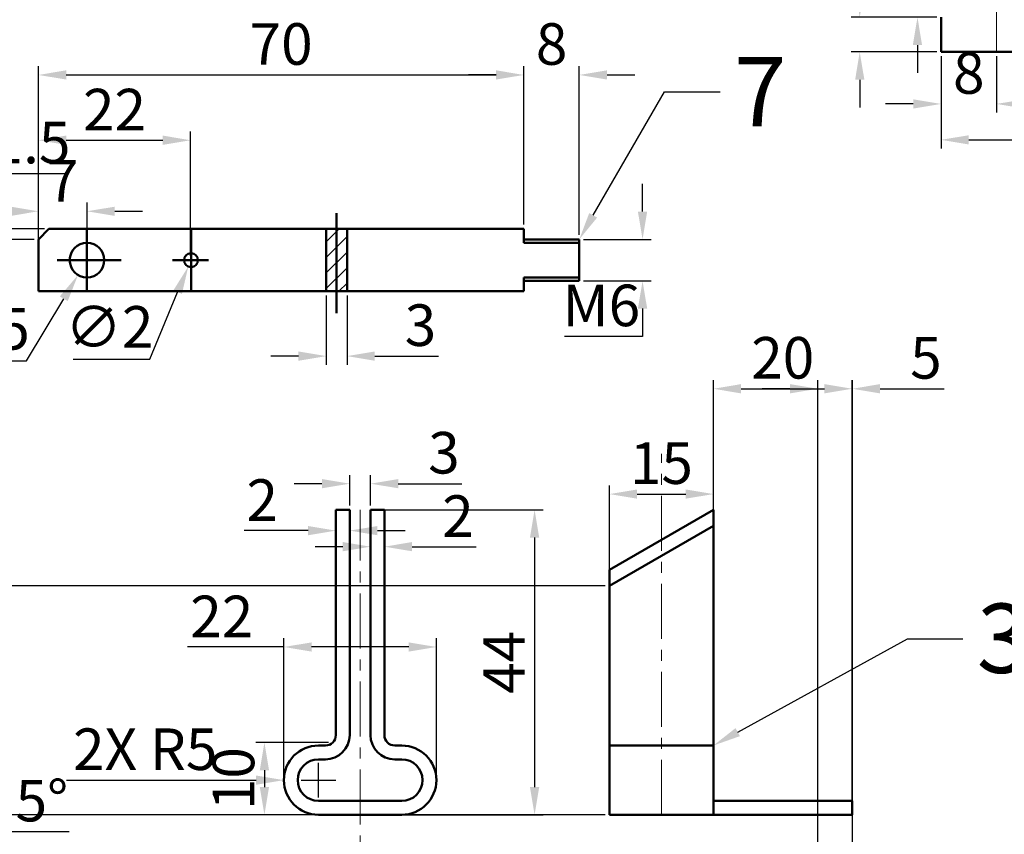
# Model space of a CAD drawing. Units: millimetres. Extents: x 1145 to 1687, y 12 to 400.
# Tile 3 of 6: x 1274 to 1416, y 168 to 285. Entities that reach past the tile are written whole.
import ezdxf
from ezdxf import colors
from ezdxf.entities.mleader import LeaderData, LeaderLine
from ezdxf.math import Vec2, Vec3

# ---------------------------------------------------------------- set-up
doc = ezdxf.new("R2010")
doc.units = ezdxf.units.MM
doc.header["$LTSCALE"] = 0.5
doc.linetypes.add('CENTER', pattern=[50.8, 31.75, -6.35, 6.35, -6.35])
for name, color, linetype, lineweight in [('M-CNTR', 1, 'CENTER', 18), ('M-DIMS', 2, 'Continuous', 25), ('M-HATC', 8, 'Continuous', 18), ('M-OUTL', 7, 'Continuous', 50), ('M-TEXT', 3, 'Continuous', 25)]:
    doc.layers.add(name, color=color, linetype=linetype, lineweight=lineweight)
doc.styles.get("Standard").update_dxf_attribs({"font": 'arial.ttf'})
doc.dimstyles.new('ISO-25', dxfattribs={"dimtxt": 6, "dimasz": 4, "dimexe": 1.25, "dimexo": 0.625, "dimtad": 1, "dimtoh": 1, "dimdec": 0, "dimtxsty": 'Standard', "dimcen": 2.5, "dimadec": 0, "dimazin": 0, "dimtfac": 1, "dimtdec": 0, "dimtofl": 0, "dimtmove": 0, "dimatfit": 3, "dimfxl": 1, "dimarcsym": 0})

# ---------------------------------------------------------------- blocks, each defined once
blk = doc.blocks.new('*D33')
at = {"layer": 'Defpoints', "color": 0, "ltscale": 0.5, "transparency": 16777216}
for p in [(1354.69, 277.15), (1346.69, 254.93), (1354.69, 253.43)]:
    blk.add_point(p, dxfattribs=at)
at = {"layer": 'M-DIMS', "color": 0, "lineweight": -2, "ltscale": 0.5, "transparency": 16777216}
for p, q in [((1346.69, 255.56), (1346.69, 278.4)), ((1354.69, 254.06), (1354.69, 278.4)), ((1342.69, 277.15), (1338.69, 277.15)), ((1358.69, 277.15), (1362.69, 277.15))]:
    blk.add_line(p, q, dxfattribs=at)
at = {"layer": 'M-DIMS', "color": 0, "ltscale": 0.5, "transparency": 16777216}
for points in [[(1342.69, 277.82), (1342.69, 276.49), (1346.69, 277.15)], [(1358.69, 277.82), (1358.69, 276.49), (1354.69, 277.15)]]:
    blk.add_solid(points, dxfattribs=at)
at = {"layer": 'M-DIMS', "color": 0, "ltscale": 0.5, "transparency": 16777216, "insert": (1350.69, 280.84), "char_height": 6, "attachment_point": 5}
blk.add_mtext('8', dxfattribs=at)
blk = doc.blocks.new('*D34')
at = {"layer": 'Defpoints', "color": 0, "ltscale": 0.5, "transparency": 16777216}
for p in [(1283.69, 257.48), (1283.69, 250.43), (1276.69, 249.68)]:
    blk.add_point(p, dxfattribs=at)
at = {"layer": 'M-DIMS', "color": 0, "lineweight": -2, "ltscale": 0.5, "transparency": 16777216}
for p, q in [((1276.69, 250.31), (1276.69, 258.73)), ((1283.69, 251.06), (1283.69, 258.73)), ((1272.69, 257.48), (1268.69, 257.48)), ((1287.69, 257.48), (1291.69, 257.48))]:
    blk.add_line(p, q, dxfattribs=at)
at = {"layer": 'M-DIMS', "color": 0, "ltscale": 0.5, "transparency": 16777216}
for points in [[(1272.69, 258.14), (1272.69, 256.81), (1276.69, 257.48)], [(1287.69, 258.14), (1287.69, 256.81), (1283.69, 257.48)]]:
    blk.add_solid(points, dxfattribs=at)
at = {"layer": 'M-DIMS', "color": 0, "ltscale": 0.5, "transparency": 16777216, "insert": (1280.19, 261.1), "char_height": 6, "attachment_point": 5}
blk.add_mtext('7', dxfattribs=at)
blk = doc.blocks.new('*D35')
at = {"layer": 'Defpoints', "color": 0, "ltscale": 0.5, "transparency": 16777216}
for p in [(1298.62, 267.73), (1298.62, 250.43), (1276.69, 249.68)]:
    blk.add_point(p, dxfattribs=at)
at = {"layer": 'M-DIMS', "color": 0, "lineweight": -2, "ltscale": 0.5, "transparency": 16777216}
for p, q in [((1276.69, 250.31), (1276.69, 268.98)), ((1298.62, 251.06), (1298.62, 268.98)), ((1280.69, 267.73), (1294.62, 267.73))]:
    blk.add_line(p, q, dxfattribs=at)
at = {"layer": 'M-DIMS', "color": 0, "ltscale": 0.5, "transparency": 16777216}
for points in [[(1280.69, 268.4), (1280.69, 267.06), (1276.69, 267.73)], [(1294.62, 268.4), (1294.62, 267.06), (1298.62, 267.73)]]:
    blk.add_solid(points, dxfattribs=at)
at = {"layer": 'M-DIMS', "color": 0, "ltscale": 0.5, "transparency": 16777216, "insert": (1287.66, 271.37), "char_height": 6, "attachment_point": 5}
blk.add_mtext('22', dxfattribs=at)
blk = doc.blocks.new('*D36')
at = {"layer": 'Defpoints', "color": 0, "ltscale": 0.5, "transparency": 16777216}
for p in [(1346.69, 277.15), (1346.69, 254.93), (1276.69, 249.68)]:
    blk.add_point(p, dxfattribs=at)
at = {"layer": 'M-DIMS', "color": 0, "lineweight": -2, "ltscale": 0.5, "transparency": 16777216}
for p, q in [((1276.69, 250.31), (1276.69, 278.4)), ((1346.69, 255.56), (1346.69, 278.4)), ((1280.69, 277.15), (1342.69, 277.15))]:
    blk.add_line(p, q, dxfattribs=at)
at = {"layer": 'M-DIMS', "color": 0, "ltscale": 0.5, "transparency": 16777216}
for points in [[(1280.69, 277.82), (1280.69, 276.49), (1276.69, 277.15)], [(1342.69, 277.82), (1342.69, 276.49), (1346.69, 277.15)]]:
    blk.add_solid(points, dxfattribs=at)
at = {"layer": 'M-DIMS', "color": 0, "ltscale": 0.5, "transparency": 16777216, "insert": (1311.69, 280.84), "char_height": 6, "attachment_point": 5}
blk.add_mtext('70', dxfattribs=at)
blk = doc.blocks.new('*D37')
at = {"layer": 'Defpoints', "color": 0, "ltscale": 0.5, "transparency": 16777216}
for p in [(1354.69, 253.43), (1354.69, 247.43), (1363.81, 247.43)]:
    blk.add_point(p, dxfattribs=at)
at = {"layer": 'M-DIMS', "color": 0, "lineweight": -2, "ltscale": 0.5, "transparency": 16777216}
for p, q in [((1363.81, 257.43), (1363.81, 261.43)), ((1355.31, 253.43), (1365.06, 253.43)), ((1355.31, 247.43), (1365.06, 247.43)), ((1363.81, 243.43), (1363.81, 239.43)), ((1363.81, 239.43), (1352.55, 239.43))]:
    blk.add_line(p, q, dxfattribs=at)
at = {"layer": 'M-DIMS', "color": 0, "ltscale": 0.5, "transparency": 16777216}
for points in [[(1363.14, 257.43), (1364.48, 257.43), (1363.81, 253.43)], [(1363.14, 243.43), (1364.48, 243.43), (1363.81, 247.43)]]:
    blk.add_solid(points, dxfattribs=at)
at = {"layer": 'M-DIMS', "color": 0, "ltscale": 0.5, "transparency": 16777216, "insert": (1357.87, 243.12), "char_height": 6, "attachment_point": 5}
blk.add_mtext('M6', dxfattribs=at)
blk = doc.blocks.new('*D38')
at = {"layer": 'Defpoints', "color": 0, "ltscale": 0.5, "transparency": 16777216}
for p in [(1318.19, 245.93), (1321.19, 245.93), (1321.19, 236.58)]:
    blk.add_point(p, dxfattribs=at)
at = {"layer": 'M-DIMS', "color": 0, "lineweight": -2, "ltscale": 0.5, "transparency": 16777216}
for p, q in [((1318.19, 245.31), (1318.19, 235.33)), ((1321.19, 245.31), (1321.19, 235.33)), ((1314.19, 236.58), (1310.19, 236.58)), ((1325.19, 236.58), (1334.37, 236.58))]:
    blk.add_line(p, q, dxfattribs=at)
at = {"layer": 'M-DIMS', "color": 0, "ltscale": 0.5, "transparency": 16777216}
for points in [[(1314.19, 237.25), (1314.19, 235.91), (1318.19, 236.58)], [(1325.19, 237.25), (1325.19, 235.91), (1321.19, 236.58)]]:
    blk.add_solid(points, dxfattribs=at)
at = {"layer": 'M-DIMS', "color": 0, "ltscale": 0.5, "transparency": 16777216, "insert": (1331.78, 240.27), "char_height": 6, "attachment_point": 5}
blk.add_mtext('3', dxfattribs=at)
blk = doc.blocks.new('*D39')
at = {"layer": 'Defpoints', "color": 0, "ltscale": 0.5, "transparency": 16777216}
for p in [(1299.07, 251.35), (1298.3, 249.51)]:
    blk.add_point(p, dxfattribs=at)
at = {"layer": 'M-DIMS', "color": 0, "lineweight": -2, "ltscale": 0.5, "transparency": 16777216}
for p, q in [((1298.69, 247.93), (1298.69, 252.93)), ((1296.19, 250.43), (1301.19, 250.43)), ((1292.74, 236.16), (1296.76, 245.82)), ((1281.71, 236.16), (1292.74, 236.16))]:
    blk.add_line(p, q, dxfattribs=at)
at = {"layer": 'M-DIMS', "color": 0, "ltscale": 0.5, "transparency": 16777216}
blk.add_solid([(1296.15, 246.07), (1297.38, 245.56), (1298.3, 249.51)], dxfattribs=at)
at = {"layer": 'M-DIMS', "color": 0, "ltscale": 0.5, "transparency": 16777216, "insert": (1286.91, 240.02), "char_height": 6, "attachment_point": 5}
blk.add_mtext('∅2', dxfattribs=at)
blk = doc.blocks.new('*D40')
at = {"layer": 'Defpoints', "color": 0, "ltscale": 0.5, "transparency": 16777216}
for p in [(1284.98, 252.57), (1282.4, 248.29)]:
    blk.add_point(p, dxfattribs=at)
at = {"layer": 'M-DIMS', "color": 0, "lineweight": -2, "ltscale": 0.5, "transparency": 16777216}
for p, q in [((1283.69, 247.93), (1283.69, 252.93)), ((1281.19, 250.43), (1286.19, 250.43)), ((1274.96, 235.89), (1280.34, 244.86)), ((1263.83, 235.89), (1274.96, 235.89))]:
    blk.add_line(p, q, dxfattribs=at)
at = {"layer": 'M-DIMS', "color": 0, "ltscale": 0.5, "transparency": 16777216}
blk.add_solid([(1279.77, 245.2), (1280.91, 244.52), (1282.4, 248.29)], dxfattribs=at)
at = {"layer": 'M-DIMS', "color": 0, "ltscale": 0.5, "transparency": 16777216, "insert": (1269.08, 239.75), "char_height": 6, "attachment_point": 5}
blk.add_mtext('∅5', dxfattribs=at)
blk = doc.blocks.new('*D41')
at = {"layer": 'Defpoints', "color": 0, "ltscale": 0.5, "transparency": 16777216}
for p in [(1406.86, 280.47), (1456.86, 280.47), (1456.86, 267.79)]:
    blk.add_point(p, dxfattribs=at)
at = {"layer": 'M-DIMS', "color": 0, "lineweight": -2, "ltscale": 0.5, "transparency": 16777216}
for p, q in [((1406.86, 279.85), (1406.86, 266.54)), ((1456.86, 279.85), (1456.86, 266.54)), ((1410.86, 267.79), (1452.86, 267.79))]:
    blk.add_line(p, q, dxfattribs=at)
at = {"layer": 'M-DIMS', "color": 0, "ltscale": 0.5, "transparency": 16777216}
for points in [[(1410.86, 268.45), (1410.86, 267.12), (1406.86, 267.79)], [(1452.86, 268.45), (1452.86, 267.12), (1456.86, 267.79)]]:
    blk.add_solid(points, dxfattribs=at)
at = {"layer": 'M-DIMS', "color": 0, "ltscale": 0.5, "transparency": 16777216, "insert": (1431.86, 271.48), "char_height": 6, "attachment_point": 5}
blk.add_mtext('50', dxfattribs=at)
blk = doc.blocks.new('*D42')
at = {"layer": 'Defpoints', "color": 0, "ltscale": 0.5, "transparency": 16777216}
for p in [(1406.86, 280.47), (1414.86, 280.47), (1414.86, 272.97)]:
    blk.add_point(p, dxfattribs=at)
at = {"layer": 'M-DIMS', "color": 0, "lineweight": -2, "ltscale": 0.5, "transparency": 16777216}
for p, q in [((1406.86, 279.85), (1406.86, 271.72)), ((1414.86, 279.85), (1414.86, 271.72)), ((1402.86, 272.97), (1398.86, 272.97)), ((1418.86, 272.97), (1422.86, 272.97))]:
    blk.add_line(p, q, dxfattribs=at)
at = {"layer": 'M-DIMS', "color": 0, "ltscale": 0.5, "transparency": 16777216}
for points in [[(1402.86, 273.63), (1402.86, 272.3), (1406.86, 272.97)], [(1418.86, 273.63), (1418.86, 272.3), (1414.86, 272.97)]]:
    blk.add_solid(points, dxfattribs=at)
at = {"layer": 'M-DIMS', "color": 0, "ltscale": 0.5, "transparency": 16777216, "insert": (1410.86, 276.66), "char_height": 6, "attachment_point": 5}
blk.add_mtext('8', dxfattribs=at)
blk = doc.blocks.new('*D43')
at = {"layer": 'Defpoints', "color": 0, "ltscale": 0.5, "transparency": 16777216}
for p in [(1395.13, 285.47), (1406.86, 285.47), (1406.86, 280.47)]:
    blk.add_point(p, dxfattribs=at)
at = {"layer": 'M-DIMS', "color": 0, "lineweight": -2, "ltscale": 0.5, "transparency": 16777216}
for p, q in [((1395.13, 289.47), (1395.13, 293.47)), ((1395.13, 293.47), (1399.74, 293.47)), ((1406.23, 285.47), (1393.88, 285.47)), ((1406.23, 280.47), (1393.88, 280.47)), ((1395.13, 276.47), (1395.13, 272.47))]:
    blk.add_line(p, q, dxfattribs=at)
at = {"layer": 'M-DIMS', "color": 0, "ltscale": 0.5, "transparency": 16777216}
for points in [[(1394.47, 289.47), (1395.8, 289.47), (1395.13, 285.47)], [(1394.47, 276.47), (1395.8, 276.47), (1395.13, 280.47)]]:
    blk.add_solid(points, dxfattribs=at)
at = {"layer": 'M-DIMS', "color": 0, "ltscale": 0.5, "transparency": 16777216, "insert": (1397.75, 297.15), "char_height": 6, "attachment_point": 5}
blk.add_mtext('5', dxfattribs=at)
blk = doc.blocks.new('*D44')
at = {"layer": 'Defpoints', "color": 0, "ltscale": 0.5, "transparency": 16777216}
for p in [(1403.46, 290.47), (1414.86, 290.47), (1406.86, 285.47)]:
    blk.add_point(p, dxfattribs=at)
at = {"layer": 'M-DIMS', "color": 0, "lineweight": -2, "ltscale": 0.5, "transparency": 16777216}
for p, q in [((1403.46, 294.47), (1403.46, 298.47)), ((1403.46, 298.47), (1408.06, 298.47)), ((1414.23, 290.47), (1402.21, 290.47)), ((1406.23, 285.47), (1402.21, 285.47)), ((1403.46, 281.47), (1403.46, 277.47))]:
    blk.add_line(p, q, dxfattribs=at)
at = {"layer": 'M-DIMS', "color": 0, "ltscale": 0.5, "transparency": 16777216}
for points in [[(1402.79, 294.47), (1404.12, 294.47), (1403.46, 290.47)], [(1402.79, 281.47), (1404.12, 281.47), (1403.46, 285.47)]]:
    blk.add_solid(points, dxfattribs=at)
at = {"layer": 'M-DIMS', "color": 0, "ltscale": 0.5, "transparency": 16777216, "insert": (1406.07, 302.15), "char_height": 6, "attachment_point": 5}
blk.add_mtext('5', dxfattribs=at)
blk = doc.blocks.new('*D60')
at = {"layer": 'Defpoints', "color": 0, "ltscale": 0.5, "transparency": 16777216}
for p in [(1324.58, 218.17), (1321.58, 214.39), (1324.58, 214.39)]:
    blk.add_point(p, dxfattribs=at)
at = {"layer": 'M-DIMS', "color": 0, "lineweight": -2, "ltscale": 0.5, "transparency": 16777216}
for p, q in [((1321.58, 215.02), (1321.58, 219.42)), ((1324.58, 215.02), (1324.58, 219.42)), ((1317.58, 218.17), (1313.58, 218.17)), ((1328.58, 218.17), (1337.75, 218.17))]:
    blk.add_line(p, q, dxfattribs=at)
at = {"layer": 'M-DIMS', "color": 0, "ltscale": 0.5, "transparency": 16777216}
for points in [[(1317.58, 218.84), (1317.58, 217.51), (1321.58, 218.17)], [(1328.58, 218.84), (1328.58, 217.51), (1324.58, 218.17)]]:
    blk.add_solid(points, dxfattribs=at)
at = {"layer": 'M-DIMS', "color": 0, "ltscale": 0.5, "transparency": 16777216, "insert": (1335.17, 221.86), "char_height": 6, "attachment_point": 5}
blk.add_mtext('3', dxfattribs=at)
blk = doc.blocks.new('*D61')
at = {"layer": 'Defpoints', "color": 0, "ltscale": 0.5, "transparency": 16777216}
for p in [(1324.58, 214.39), (1326.58, 214.39), (1326.58, 209.08)]:
    blk.add_point(p, dxfattribs=at)
at = {"layer": 'M-DIMS', "color": 0, "lineweight": -2, "ltscale": 0.5, "transparency": 16777216}
for p, q in [((1324.58, 213.77), (1324.58, 207.83)), ((1326.58, 213.77), (1326.58, 207.83)), ((1320.58, 209.08), (1316.58, 209.08)), ((1330.58, 209.08), (1339.8, 209.08))]:
    blk.add_line(p, q, dxfattribs=at)
at = {"layer": 'M-DIMS', "color": 0, "ltscale": 0.5, "transparency": 16777216}
for points in [[(1320.58, 209.75), (1320.58, 208.42), (1324.58, 209.08)], [(1330.58, 209.75), (1330.58, 208.42), (1326.58, 209.08)]]:
    blk.add_solid(points, dxfattribs=at)
at = {"layer": 'M-DIMS', "color": 0, "ltscale": 0.5, "transparency": 16777216, "insert": (1337.19, 212.72), "char_height": 6, "attachment_point": 5}
blk.add_mtext('2', dxfattribs=at)
blk = doc.blocks.new('*D62')
at = {"layer": 'Defpoints', "color": 0, "ltscale": 0.5, "transparency": 16777216}
for p in [(1319.58, 214.39), (1321.58, 214.39), (1321.58, 211.4)]:
    blk.add_point(p, dxfattribs=at)
at = {"layer": 'M-DIMS', "color": 0, "lineweight": -2, "ltscale": 0.5, "transparency": 16777216}
for p, q in [((1319.58, 213.77), (1319.58, 210.15)), ((1321.58, 213.77), (1321.58, 210.15)), ((1315.58, 211.4), (1306.35, 211.4)), ((1325.58, 211.4), (1329.58, 211.4))]:
    blk.add_line(p, q, dxfattribs=at)
at = {"layer": 'M-DIMS', "color": 0, "ltscale": 0.5, "transparency": 16777216}
for points in [[(1315.58, 212.06), (1315.58, 210.73), (1319.58, 211.4)], [(1325.58, 212.06), (1325.58, 210.73), (1321.58, 211.4)]]:
    blk.add_solid(points, dxfattribs=at)
at = {"layer": 'M-DIMS', "color": 0, "ltscale": 0.5, "transparency": 16777216, "insert": (1308.96, 215.03), "char_height": 6, "attachment_point": 5}
blk.add_mtext('2', dxfattribs=at)
blk = doc.blocks.new('*D63')
at = {"layer": 'Defpoints', "color": 0, "ltscale": 0.5, "transparency": 16777216}
for p in [(1319.14, 180.83), (1309.28, 170.39), (1319.14, 170.39)]:
    blk.add_point(p, dxfattribs=at)
at = {"layer": 'M-DIMS', "color": 0, "lineweight": -2, "ltscale": 0.5, "transparency": 16777216}
for p, q in [((1318.51, 180.83), (1308.03, 180.83)), ((1309.28, 176.83), (1309.28, 174.39)), ((1318.51, 170.39), (1308.03, 170.39))]:
    blk.add_line(p, q, dxfattribs=at)
at = {"layer": 'M-DIMS', "color": 0, "ltscale": 0.5, "transparency": 16777216}
for points in [[(1308.61, 176.83), (1309.94, 176.83), (1309.28, 180.83)], [(1308.61, 174.39), (1309.94, 174.39), (1309.28, 170.39)]]:
    blk.add_solid(points, dxfattribs=at)
at = {"layer": 'M-DIMS', "color": 0, "ltscale": 0.5, "transparency": 16777216, "insert": (1305.59, 175.61), "char_height": 6, "attachment_point": 5, "rotation": 90}
blk.add_mtext('10', dxfattribs=at)
blk = doc.blocks.new('*D64')
at = {"layer": 'Defpoints', "color": 0, "ltscale": 0.5, "transparency": 16777216}
for p in [(1334.08, 194.61), (1312.08, 175.39), (1334.08, 175.39)]:
    blk.add_point(p, dxfattribs=at)
at = {"layer": 'M-DIMS', "color": 0, "lineweight": -2, "ltscale": 0.5, "transparency": 16777216}
for p, q in [((1312.08, 194.61), (1298.19, 194.61)), ((1312.08, 176.02), (1312.08, 195.86)), ((1330.08, 194.61), (1316.08, 194.61)), ((1334.08, 176.02), (1334.08, 195.86))]:
    blk.add_line(p, q, dxfattribs=at)
at = {"layer": 'M-DIMS', "color": 0, "ltscale": 0.5, "transparency": 16777216}
for points in [[(1316.08, 195.27), (1316.08, 193.94), (1312.08, 194.61)], [(1330.08, 195.27), (1330.08, 193.94), (1334.08, 194.61)]]:
    blk.add_solid(points, dxfattribs=at)
at = {"layer": 'M-DIMS', "color": 0, "ltscale": 0.5, "transparency": 16777216, "insert": (1303.13, 198.24), "char_height": 6, "attachment_point": 5}
blk.add_mtext('22', dxfattribs=at)
blk = doc.blocks.new('*D71')
at = {"layer": 'Defpoints', "color": 0, "ltscale": 0.5, "transparency": 16777216}
for p in [(1325.58, 214.39), (1323.08, 170.39), (1348.24, 170.39)]:
    blk.add_point(p, dxfattribs=at)
at = {"layer": 'M-DIMS', "color": 0, "lineweight": -2, "ltscale": 0.5, "transparency": 16777216}
for p, q in [((1326.2, 214.39), (1349.49, 214.39)), ((1348.24, 210.39), (1348.24, 174.39)), ((1323.7, 170.39), (1349.49, 170.39))]:
    blk.add_line(p, q, dxfattribs=at)
at = {"layer": 'M-DIMS', "color": 0, "ltscale": 0.5, "transparency": 16777216}
for points in [[(1347.57, 210.39), (1348.91, 210.39), (1348.24, 214.39)], [(1347.57, 174.39), (1348.91, 174.39), (1348.24, 170.39)]]:
    blk.add_solid(points, dxfattribs=at)
at = {"layer": 'M-DIMS', "color": 0, "ltscale": 0.5, "transparency": 16777216, "insert": (1344.61, 192.39), "char_height": 6, "attachment_point": 5, "rotation": 90}
blk.add_mtext('44', dxfattribs=at)
blk = doc.blocks.new('*D72')
at = {"layer": 'Defpoints', "color": 0, "ltscale": 0.5, "transparency": 16777216}
for p in [(1374.03, 216.67), (1359.03, 203.42), (1374.03, 203.42)]:
    blk.add_point(p, dxfattribs=at)
at = {"layer": 'M-DIMS', "color": 0, "lineweight": -2, "ltscale": 0.5, "transparency": 16777216}
for p, q in [((1359.03, 204.05), (1359.03, 217.92)), ((1374.03, 204.05), (1374.03, 217.92)), ((1363.03, 216.67), (1370.03, 216.67))]:
    blk.add_line(p, q, dxfattribs=at)
at = {"layer": 'M-DIMS', "color": 0, "ltscale": 0.5, "transparency": 16777216}
for points in [[(1363.03, 217.34), (1363.03, 216.01), (1359.03, 216.67)], [(1370.03, 217.34), (1370.03, 216.01), (1374.03, 216.67)]]:
    blk.add_solid(points, dxfattribs=at)
at = {"layer": 'M-DIMS', "color": 0, "ltscale": 0.5, "transparency": 16777216, "insert": (1366.53, 220.36), "char_height": 6, "attachment_point": 5}
blk.add_mtext('15', dxfattribs=at)
blk = doc.blocks.new('*D73')
at = {"layer": 'Defpoints', "color": 0, "ltscale": 0.5, "transparency": 16777216}
for p in [(1255.04, 170.27), (1252.07, 167.52), (1257.42, 156.31), (1252.07, 136.31), (1252.07, 136.31)]:
    blk.add_point(p, dxfattribs=at)
at = {"layer": 'M-DIMS', "color": 0, "lineweight": -2, "ltscale": 0.5, "transparency": 16777216}
for p, q in [((1252.07, 168.14), (1252.07, 171.65)), ((1257.59, 156.91), (1261.21, 170.44)), ((1264.68, 167.98), (1281.14, 167.98))]:
    blk.add_line(p, q, dxfattribs=at)
for start, end in [(81.7274, 83.2726), (68.2726, 75)]:
    blk.add_arc((1252.07, 136.31), 34.09, start, end, dxfattribs=at)
at = {"layer": 'M-DIMS', "color": 0, "ltscale": 0.5, "transparency": 16777216}
for points in [[(1256.02, 169.5), (1256.1, 170.83), (1252.07, 170.4)], [(1257.1, 170.69), (1256.84, 169.39), (1260.89, 169.24)]]:
    blk.add_solid(points, dxfattribs=at)
at = {"layer": 'M-DIMS', "color": 0, "ltscale": 0.5, "transparency": 16777216, "insert": (1274.91, 171.66), "char_height": 6, "attachment_point": 5}
blk.add_mtext('15°', dxfattribs=at)
blk = doc.blocks.new('CONTACT-CLIP')
at = {"ltscale": 0.5}
for p, q in [((7.5, 11.5), (7.5, 44)), ((7.5, 44), (9.5, 44)), ((9.5, 11.5), (9.5, 44)), ((12.5, 11.5), (12.5, 44)), ((12.5, 44), (14.5, 44)), ((14.5, 11.5), (14.5, 44)), ((5, 10), (6, 10)), ((5, 2), (17, 2)), ((5, 0), (17, 0))]:
    blk.add_line(p, q, dxfattribs=at)
for centre, radius, start, end in [((6, 11.5), 1.5, 270, 0), ((6, 11.5), 3.5, 270, 0), ((16, 11.5), 3.5, 180, 270), ((16, 11.5), 1.5, 180, 270), ((5, 5), 5, 90, 270), ((17, 5), 5, 270, 90), ((5, 5), 3, 90, 270), ((17, 5), 3, 270, 90)]:
    blk.add_arc(centre, radius, start, end, dxfattribs=at)
for points in [[(16, 10), (16.33, 10), (16.67, 10), (17, 10)], [(6, 8), (5.67, 8), (5.33, 8), (5, 8)], [(16, 8), (16.33, 8), (16.67, 8), (17, 8)]]:
    blk.add_open_spline(points, degree=3)
blk = doc.blocks.new('BRACKET')
at = {"ltscale": 0.5}
for p, q in [((15, 44), (0, 35.34)), ((15, 44), (15, 30)), ((0, 30), (0, 35.34)), ((0, 30), (0, 0)), ((15, 0), (15, 30)), ((35, 2), (15, 2)), ((35, 0), (35, 2)), ((0, 0), (15, 0)), ((15, 0), (35, 0))]:
    blk.add_line(p, q, dxfattribs=at)
blk = doc.blocks.new('*D98')
at = {"layer": 'Defpoints', "color": 0, "ltscale": 0.5, "transparency": 16777216}
for p in [(1394.07, 231.87), (1394.07, 156.31), (1389.07, 146.81)]:
    blk.add_point(p, dxfattribs=at)
at = {"layer": 'M-DIMS', "color": 0, "lineweight": -2, "ltscale": 0.5, "transparency": 16777216}
for p, q in [((1389.07, 147.44), (1389.07, 233.12)), ((1394.07, 156.94), (1394.07, 233.12)), ((1385.07, 231.87), (1381.07, 231.87)), ((1398.07, 231.87), (1407.29, 231.87))]:
    blk.add_line(p, q, dxfattribs=at)
at = {"layer": 'M-DIMS', "color": 0, "ltscale": 0.5, "transparency": 16777216}
for points in [[(1385.07, 232.54), (1385.07, 231.2), (1389.07, 231.87)], [(1398.07, 232.54), (1398.07, 231.2), (1394.07, 231.87)]]:
    blk.add_solid(points, dxfattribs=at)
at = {"layer": 'M-DIMS', "color": 0, "ltscale": 0.5, "transparency": 16777216, "insert": (1404.68, 235.55), "char_height": 6, "attachment_point": 5}
blk.add_mtext('5', dxfattribs=at)
blk = doc.blocks.new('*D99')
at = {"layer": 'Defpoints', "color": 0, "ltscale": 0.5, "transparency": 16777216}
for p in [(1394.03, 231.87), (1374.03, 170.39), (1394.03, 170.39)]:
    blk.add_point(p, dxfattribs=at)
at = {"layer": 'M-DIMS', "color": 0, "lineweight": -2, "ltscale": 0.5, "transparency": 16777216}
for p, q in [((1374.03, 171.02), (1374.03, 233.12)), ((1394.03, 171.02), (1394.03, 233.12)), ((1378.03, 231.87), (1390.03, 231.87))]:
    blk.add_line(p, q, dxfattribs=at)
at = {"layer": 'M-DIMS', "color": 0, "ltscale": 0.5, "transparency": 16777216}
for points in [[(1378.03, 232.54), (1378.03, 231.2), (1374.03, 231.87)], [(1390.03, 232.54), (1390.03, 231.2), (1394.03, 231.87)]]:
    blk.add_solid(points, dxfattribs=at)
at = {"layer": 'M-DIMS', "color": 0, "ltscale": 0.5, "transparency": 16777216, "insert": (1384.03, 235.56), "char_height": 6, "attachment_point": 5}
blk.add_mtext('20', dxfattribs=at)
blk = doc.blocks.new('*D100')
at = {"layer": 'Defpoints', "color": 0, "ltscale": 0.5, "transparency": 16777216}
for p in [(1230.63, 203.42), (1359.03, 203.42), (1359.03, 170.39)]:
    blk.add_point(p, dxfattribs=at)
at = {"layer": 'M-DIMS', "color": 0, "lineweight": -2, "ltscale": 0.5, "transparency": 16777216}
for p, q in [((1358.41, 203.42), (1229.38, 203.42)), ((1230.63, 174.39), (1230.63, 199.42)), ((1358.41, 170.39), (1229.38, 170.39))]:
    blk.add_line(p, q, dxfattribs=at)
at = {"layer": 'M-DIMS', "color": 0, "ltscale": 0.5, "transparency": 16777216}
for points in [[(1229.96, 199.42), (1231.29, 199.42), (1230.63, 203.42)], [(1229.96, 174.39), (1231.29, 174.39), (1230.63, 170.39)]]:
    blk.add_solid(points, dxfattribs=at)
at = {"layer": 'M-DIMS', "color": 0, "ltscale": 0.5, "transparency": 16777216, "insert": (1226.94, 186.91), "char_height": 6, "attachment_point": 5, "rotation": 90}
blk.add_mtext('33.03', dxfattribs=at)
blk = doc.blocks.new('*D101')
at = {"layer": 'Defpoints', "color": 0, "ltscale": 0.5, "transparency": 16777216}
for p in [(1269.79, 254.93), (1278.19, 254.93), (1276.69, 253.43)]:
    blk.add_point(p, dxfattribs=at)
at = {"layer": 'M-DIMS', "color": 0, "lineweight": -2, "ltscale": 0.5, "transparency": 16777216}
for p, q in [((1269.79, 258.93), (1269.79, 262.93)), ((1269.79, 262.93), (1280.82, 262.93)), ((1277.56, 254.93), (1268.54, 254.93)), ((1276.06, 253.43), (1268.54, 253.43)), ((1269.79, 249.43), (1269.79, 245.43))]:
    blk.add_line(p, q, dxfattribs=at)
at = {"layer": 'M-DIMS', "color": 0, "ltscale": 0.5, "transparency": 16777216}
for points in [[(1269.12, 258.93), (1270.46, 258.93), (1269.79, 254.93)], [(1269.12, 249.43), (1270.46, 249.43), (1269.79, 253.43)]]:
    blk.add_solid(points, dxfattribs=at)
at = {"layer": 'M-DIMS', "color": 0, "ltscale": 0.5, "transparency": 16777216, "insert": (1275.62, 266.62), "char_height": 6, "attachment_point": 5}
blk.add_mtext('1.5', dxfattribs=at)
blk = doc.blocks.new('*D118')
at = {"layer": 'Defpoints', "color": 0, "ltscale": 0.5, "transparency": 16777216}
for p in [(1312.08, 175.39), (1317.08, 175.39)]:
    blk.add_point(p, dxfattribs=at)
at = {"layer": 'M-DIMS', "color": 0, "lineweight": -2, "ltscale": 0.5, "transparency": 16777216}
for p, q in [((1317.08, 172.89), (1317.08, 177.89)), ((1280.74, 175.39), (1304.08, 175.39)), ((1304.08, 175.39), (1308.08, 175.39)), ((1314.58, 175.39), (1319.58, 175.39))]:
    blk.add_line(p, q, dxfattribs=at)
at = {"layer": 'M-DIMS', "color": 0, "ltscale": 0.5, "transparency": 16777216}
blk.add_solid([(1308.08, 176.06), (1308.08, 174.73), (1312.08, 175.39)], dxfattribs=at)
at = {"layer": 'M-DIMS', "color": 0, "ltscale": 0.5, "transparency": 16777216, "insert": (1292.09, 179.08), "char_height": 6, "attachment_point": 5}
blk.add_mtext('2X R5', dxfattribs=at)

msp = doc.modelspace()

# ---------------------------------------------------------------- hatches: boundary and pattern name
at = {"layer": 'M-HATC', "ltscale": 0.5}
h = msp.add_hatch(dxfattribs=at)
h.set_pattern_fill('ANSI31', color=256, scale=0.5)
h.set_pattern_definition([(45, (528.9489, -64.7), (-1.122532, 1.122532), [])])
h.paths.add_polyline_path([(1321.1892, 254.9307), (1319.6892, 254.9307), (1319.6892, 245.9307), (1321.1892, 245.9307)])
h.paths.add_polyline_path([(1319.6892, 254.9307), (1318.1892, 254.9307), (1318.1892, 245.9307), (1319.6892, 245.9307)])

# ---------------------------------------------------------------- linework, layer by layer
at = {"layer": 'M-CNTR', "ltscale": 0.5}
for p, q in [((1414.8568, 280.4724), (1414.8568, 294.0648)), ((1366.5331, 170.3937), (1366.5331, 222.471)), ((1323.0658, 156.3102), (1323.0755, 214.3937))]:
    msp.add_line(p, q, dxfattribs=at)
at = {"layer": 'M-OUTL', "ltscale": 0.5}
for p, q in [((1406.8568, 285.4724), (1406.8568, 280.4724)), ((1406.8568, 280.4724), (1456.8568, 280.4724)), ((1319.6892, 242.7615), (1319.6892, 257.1856)), ((1276.6892, 253.4307), (1278.1892, 254.9307)), ((1278.1892, 254.9307), (1346.6892, 254.9307)), ((1283.6892, 245.9307), (1283.6892, 254.9307)), ((1298.6892, 245.9307), (1298.6892, 254.9307)), ((1318.1892, 245.9307), (1318.1892, 254.9307)), ((1321.1892, 245.9307), (1321.1892, 254.9307)), ((1346.6892, 253.4307), (1346.6892, 254.9307)), ((1346.6892, 252.9307), (1346.6892, 254.1807)), ((1276.6892, 245.9307), (1276.6892, 253.4307)), ((1346.6892, 253.4307), (1354.6892, 253.4307)), ((1346.6892, 252.9307), (1354.6892, 252.9307)), ((1354.6892, 253.4307), (1354.6892, 247.4307)), ((1279.3722, 250.4307), (1288.6304, 250.4307)), ((1296.0094, 250.4307), (1301.2344, 250.4307)), ((1354.6892, 247.9307), (1346.6892, 247.9307)), ((1346.6892, 247.9307), (1346.6892, 245.9307)), ((1346.6892, 245.9307), (1346.6892, 247.4307)), ((1354.6892, 247.4307), (1346.6892, 247.4307)), ((1276.6892, 245.9307), (1346.6892, 245.9307)), ((1374.0331, 212.0843), (1359.0331, 203.424)), ((1359.0331, 180.3937), (1374.0331, 180.3937))]:
    msp.add_line(p, q, dxfattribs=at)
for centre, radius in [((1283.6892, 250.4307), 2.5), ((1298.6892, 250.4307), 1)]:
    msp.add_circle(centre, radius, dxfattribs=at)

# ---------------------------------------------------------------- block references
at = {"layer": 'M-OUTL'}
for name, p in [('CONTACT-CLIP', (1312.0759, 170.3941)), ('BRACKET', (1359.033, 170.394))]:
    msp.add_blockref(name, p, dxfattribs=at)

# ---------------------------------------------------------------- dimensions: what is measured, and where the dimension line sits
at = {"layer": 'M-DIMS', "ltscale": 0.5}
for base, p1, p2, override, picture, middle in [((1403.4572, 290.4724), (1406.8568, 285.4724), (1414.8568, 290.4724), {"dimclrd": 0, "dimclre": 0, "dimclrt": 0}, '*D44', (1406.0712, 302.1485)), ((1395.1331, 285.4724), (1406.8568, 280.4724), (1406.8568, 285.4724), {"dimclrd": 0, "dimclre": 0, "dimclrt": 0}, '*D43', (1397.7472, 297.1485)), ((1269.7892, 254.9307), (1276.6892, 253.4307), (1278.1892, 254.9307), {"dimdec": 1, "dimlfac": 1, "dimrnd": 0, "dimzin": 0, "dimdsep": 46, "dimlunit": 2}, '*D101', (1275.6161, 266.6191)), ((1348.2384, 170.3937), (1325.5755, 214.3937), (1323.0755, 170.3937), {"dimclrd": 0, "dimclre": 0, "dimclrt": 0}, '*D71', (1344.6134, 192.3937)), ((1230.6278, 203.424), (1359.0331, 170.3937), (1359.0331, 203.424), {"dimdec": 2, "dimlfac": 1, "dimrnd": 0, "dimzin": 0, "dimdsep": 46, "dimlunit": 2}, '*D100', (1226.9373, 186.9089)), ((1309.2765, 170.3937), (1319.1362, 180.833), (1319.1362, 170.3937), {"dimclrd": 0, "dimclre": 0, "dimclrt": 0}, '*D63', (1305.5881, 175.6134))]:
    dim = msp.add_linear_dim(base=base, p1=p1, p2=p2, angle=90, dimstyle='ISO-25', override=override, dxfattribs=at)
    dim.commit()
    dim.dimension.update_dxf_attribs({"geometry": picture, "text_midpoint": middle})
for base, p1, p2, picture, middle in [((1346.6892, 277.1536), (1276.6892, 249.6807), (1346.6892, 254.9307), '*D36', (1311.6892, 277.1536)), ((1354.6892, 277.1548), (1346.6892, 254.9307), (1354.6892, 253.4307), '*D33', (1350.6892, 277.1548)), ((1456.8568, 267.7873), (1406.8568, 280.4724), (1456.8568, 280.4724), '*D41', (1431.8568, 267.7873)), ((1298.6219, 267.7288), (1276.6892, 249.6807), (1298.6219, 250.4307), '*D35', (1287.6555, 267.7288)), ((1283.6892, 257.4758), (1276.6892, 249.6807), (1283.6892, 250.4307), '*D34', (1280.1892, 257.4758)), ((1321.5755, 211.3958), (1319.5755, 214.3937), (1321.5755, 214.3937), '*D62', (1308.9635, 211.3958)), ((1334.0755, 194.6065), (1312.0755, 175.3937), (1334.0755, 175.3937), '*D64', (1303.1326, 194.6065))]:
    dim = msp.add_linear_dim(base=base, p1=p1, p2=p2, dimstyle='ISO-25', override={"dimclrd": 0, "dimclre": 0, "dimclrt": 0}, dxfattribs=at)
    dim.commit()
    dim.dimension.update_dxf_attribs({"geometry": picture, "text_midpoint": middle, "dimtype": 160})
for base, p1, p2, override, picture, middle in [((1414.8568, 272.9677), (1406.8568, 280.4724), (1414.8568, 280.4724), {"dimclrd": 0, "dimclre": 0, "dimclrt": 0}, '*D42', (1410.8568, 276.6561)), ((1321.1892, 236.5787), (1318.1892, 245.9307), (1321.1892, 245.9307), {"dimclrd": 0, "dimclre": 0, "dimclrt": 0}, '*D38', (1331.7787, 240.2692)), ((1394.0331, 231.871), (1374.0331, 170.3937), (1394.0331, 170.3937), {"dimdec": 0, "dimlfac": 1, "dimrnd": 0, "dimzin": 0, "dimdsep": 46, "dimlunit": 2}, '*D99', (1384.0331, 235.5594)), ((1394.0658, 231.871), (1389.0658, 146.8102), (1394.0658, 156.3102), {"dimdec": 0, "dimlfac": 1, "dimrnd": 0, "dimzin": 0, "dimdsep": 46, "dimlunit": 2}, '*D98', (1404.6799, 235.5471)), ((1324.5755, 218.1742), (1321.5755, 214.3937), (1324.5755, 214.3937), {"dimclrd": 0, "dimclre": 0, "dimclrt": 0}, '*D60', (1335.165, 221.8647)), ((1374.0331, 216.6745), (1359.0331, 203.424), (1374.0331, 203.424), {"dimclrd": 0, "dimclre": 0, "dimclrt": 0}, '*D72', (1366.5331, 220.363)), ((1326.5755, 209.085), (1324.5755, 214.3937), (1326.5755, 214.3937), {"dimclrd": 0, "dimclre": 0, "dimclrt": 0}, '*D61', (1337.1875, 212.7223))]:
    dim = msp.add_linear_dim(base=base, p1=p1, p2=p2, dimstyle='ISO-25', override=override, dxfattribs=at)
    dim.commit()
    dim.dimension.update_dxf_attribs({"geometry": picture, "text_midpoint": middle})
dim = msp.add_linear_dim(base=(1363.8102, 247.4307), p1=(1354.6892, 253.4307), p2=(1354.6892, 247.4307), angle=90, text='M<>', dimstyle='ISO-25', override={"dimclrd": 0, "dimclre": 0, "dimclrt": 0}, dxfattribs=at)
dim.commit()
dim.dimension.update_dxf_attribs({"geometry": '*D37', "text_midpoint": (1357.8666, 243.1191)})
for p1, p2, picture, middle in [((1284.9763, 252.5739), (1282.4021, 248.2874), '*D40', (1269.0781, 239.7452)), ((1299.0741, 251.3536), (1298.3042, 249.5077), '*D39', (1286.9116, 240.0162))]:
    dim = msp.add_diameter_dim_2p(p1=p1, p2=p2, dimstyle='ISO-25', override={"dimclrd": 0, "dimclre": 0, "dimclrt": 0}, dxfattribs=at)
    dim.commit()
    dim.dimension.update_dxf_attribs({"geometry": picture, "text_midpoint": middle})
dim = msp.add_radius_dim(center=(1317.0755, 175.3937), mpoint=(1312.0755, 175.394), text='2X <>', dimstyle='ISO-25', override={"dimdec": 0, "dimlfac": 1, "dimrnd": 0, "dimzin": 0, "dimdsep": 46, "dimlunit": 2}, dxfattribs=at)
dim.commit()
dim.dimension.update_dxf_attribs({"geometry": '*D118', "text_midpoint": (1292.0931, 179.0829)})
dim = msp.add_angular_dim_2l(base=(1255.0366, 170.267), line1=((1252.0658, 136.3102), (1257.4248, 156.3102)), line2=((1252.0658, 136.3102), (1252.0658, 167.5151)), dimstyle='ISO-25', override={"dimclrd": 0, "dimclre": 0, "dimclrt": 0}, dxfattribs=at)
dim.commit()
dim.dimension.update_dxf_attribs({"geometry": '*D73', "text_midpoint": (1274.9123, 171.6634)})

# ---------------------------------------------------------------- leaders
at = {"layer": 'M-TEXT', "ltscale": 0.5}
ml = msp.add_multileader_mtext('Standard', dxfattribs=at)
ml.set_content('7', color=256)
ml.set_leader_properties()
ml.build(insert=Vec2(0, 0))
ctx = ml.context
ctx.base_point, ctx.char_height, ctx.plane_origin = Vec3(1374.9879, 274.7327), 10, Vec3(1354.6892, 253.4307)
notes = []
notes.append((ctx, [(0, (1, 1, 0), (1366.9879, 274.7327), (1, 0), 8, [(0, [(1354.6892, 253.4307)], 0, [])])]))
ctx.mtext.insert, ctx.mtext.flow_direction = Vec3(1376.9879, 279.7327), 5
ml = msp.add_multileader_mtext('Standard', dxfattribs=at)
ml.set_content('3', color=256)
ml.set_leader_properties()
ml.build(insert=Vec2(0, 0))
ctx = ml.context
ctx.base_point, ctx.char_height, ctx.plane_origin = Vec3(1410.0231, 195.7757), 10, Vec3(1379.2377, 156.3102)
notes.append((ctx, [(0, (1, 1, 0), (1402.0231, 195.7757), (1, 0), 8, [(0, [(1374.0331, 180.3937)], 0, [])])]))
ctx.mtext.insert, ctx.mtext.flow_direction = Vec3(1412.0231, 200.8644), 5
for ctx, leaders in notes:
    for number, flags, end, landing, length, lines in leaders:
        leader = LeaderData()
        leader.index, (leader.has_last_leader_line, leader.has_dogleg_vector, leader.attachment_direction) = number, flags
        leader.last_leader_point, leader.dogleg_vector, leader.dogleg_length = Vec3(end), Vec3(landing), length
        for number, points, colour, breaks in lines:
            line = LeaderLine()
            line.index, line.vertices, line.color, line.breaks = number, Vec3.list(points), colors.encode_raw_color(colour), breaks
            leader.lines.append(line)
        ctx.leaders.append(leader)

doc.saveas('drawing.dxf')
